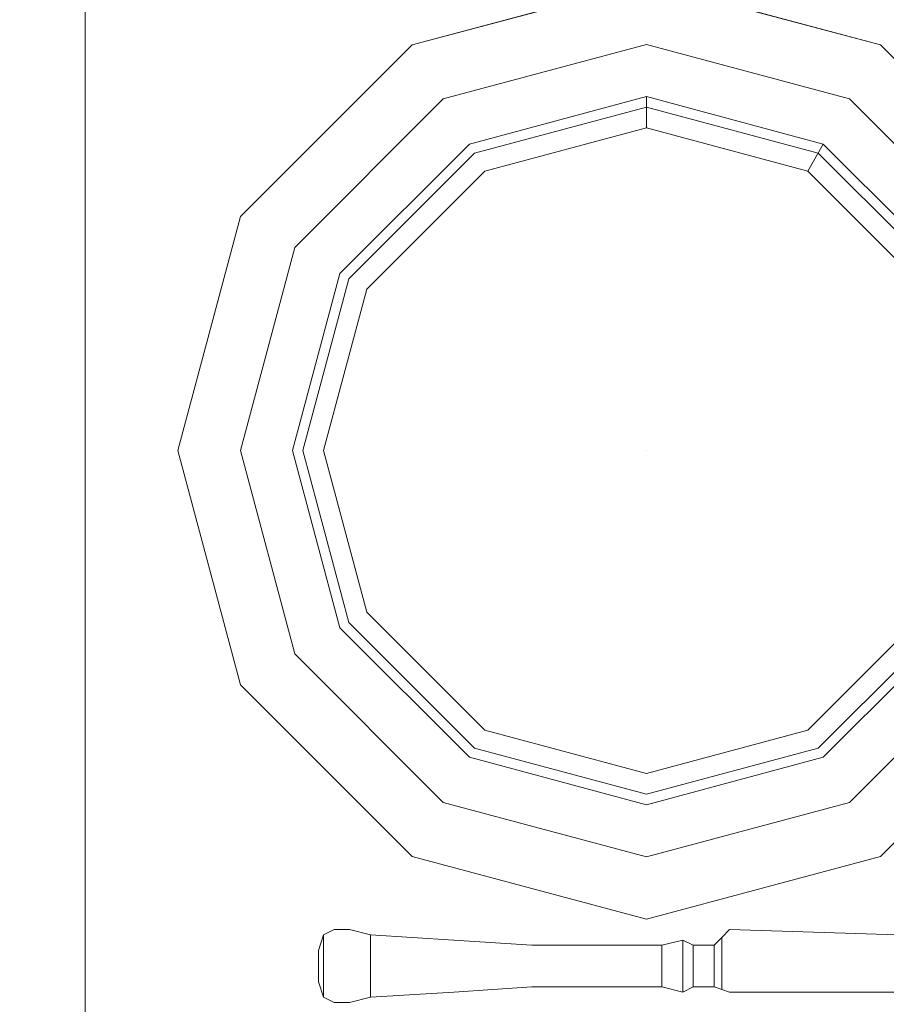
# Model space of a CAD drawing. Units: inches. Extents: x 375 to 1122, y 27 to 1069.
# Tile 38 of 155: x 705.14 to 715.39, y 296.54 to 308.18. Entities that reach past the tile are written whole.
import ezdxf

# ---------------------------------------------------------------- set-up
doc = ezdxf.new("R2010")
doc.units = ezdxf.units.IN
doc.layers.add('A-ANNO-DIMS', color=2, linetype='Continuous', lineweight=18)
doc.layers.add('Furniture', color=30, linetype='Continuous', lineweight=18)
doc.styles.get("Standard").update_dxf_attribs({"font": 'arial.ttf'})
doc.dimstyles.new('ISO-25', dxfattribs={"dimtxt": 12, "dimasz": 2.5, "dimexe": 1.5, "dimexo": 1.5, "dimtad": 1, "dimdec": 1, "dimlunit": 3, "dimtxsty": 'Standard', "dimblk": 'ARCHTICK', "dimcen": 2.5, "dimadec": 0, "dimazin": 0, "dimtfac": 1, "dimtdec": 1, "dimtmove": 0, "dimatfit": 3, "dimfxl": 1.5, "dimfxlon": 1, "dimarcsym": 0})

# ---------------------------------------------------------------- blocks, each defined once
blk = doc.blocks.new('A$C403C54AD')
blk.add_line((0.83575, 0.52421, -0.0006), (1.99923, 0.52421, -0.0006))
at = {"linetype": 'ByBlock'}
for points, invisible_edges in [([(1.01094, 0.81008, -0.00874), (1.02018, 0.79408, -0.00874), (0.97623, 0.75014, -0.00874), (0.96024, 0.75938, -0.00874)], 5), ([(1.02787, 0.78075, -0.02259), (1.01094, 0.81008, -0.01335), (0.96024, 0.75938, -0.01335), (0.98956, 0.74244, -0.02259)], 5), ([(1.17085, 0.74244, -0.02259), (1.20017, 0.75938, -0.01335), (1.14947, 0.81008, -0.01335), (1.13254, 0.78075, -0.02259)], 5), ([(1.20017, 0.75938, -0.00874), (1.18418, 0.75014, -0.00874), (1.14023, 0.79408, -0.00874), (1.14947, 0.81008, -0.00874)], 5), ([(1.02018, 0.79408, -0.00874), (1.02941, 0.77809, -0.01489), (0.99223, 0.74091, -0.01489), (0.97623, 0.75014, -0.00874)], 5), ([(1.18418, 0.75014, -0.00874), (1.16818, 0.74091, -0.01489), (1.131, 0.77809, -0.01489), (1.14023, 0.79408, -0.00874)], 5), ([(1.0802, 0.7917, -0.01489), (1.0802, 0.69011, -0.01489), (1.0802, 0.69011, -0.01489), (1.02941, 0.77809, -0.01489)], 5), ([(1.131, 0.77809, -0.01489), (1.0802, 0.69011, -0.01489), (1.0802, 0.69011, -0.01489), (1.0802, 0.7917, -0.01489)], 5), ([(1.03249, 0.77276, -0.03183), (1.02787, 0.78075, -0.02259), (0.98956, 0.74244, -0.02259), (0.99756, 0.73783, -0.03183)], 1), ([(1.16285, 0.73783, -0.03183), (1.17085, 0.74244, -0.02259), (1.13254, 0.78075, -0.02259), (1.12792, 0.77276, -0.03183)], 5), ([(1.02941, 0.77809, -0.01489), (1.0802, 0.69011, -0.01489), (1.0802, 0.69011, -0.01489), (0.99223, 0.74091, -0.01489)], 5), ([(1.16818, 0.74091, -0.01489), (1.0802, 0.69011, -0.01489), (1.0802, 0.69011, -0.01489), (1.131, 0.77809, -0.01489)], 5), ([(0.96024, 0.75938, -0.00874), (0.97623, 0.75014, -0.00874), (0.96015, 0.69011, -0.00874), (0.94168, 0.69011, -0.00874)], 5), ([(0.98956, 0.74244, -0.02259), (0.96024, 0.75938, -0.01335), (0.94168, 0.69011, -0.01335), (0.97554, 0.69011, -0.02259)], 5), ([(1.18487, 0.69011, -0.02259), (1.21873, 0.69011, -0.01335), (1.20017, 0.75938, -0.01335), (1.17085, 0.74244, -0.02259)], 5), ([(1.21873, 0.69011, -0.00874), (1.20026, 0.69011, -0.00874), (1.18418, 0.75014, -0.00874), (1.20017, 0.75938, -0.00874)], 5), ([(0.97623, 0.75014, -0.00874), (0.99223, 0.74091, -0.01489), (0.97862, 0.69011, -0.01489), (0.96015, 0.69011, -0.00874)], 5), ([(1.20026, 0.69011, -0.00874), (1.18179, 0.69011, -0.01489), (1.16818, 0.74091, -0.01489), (1.18418, 0.75014, -0.00874)], 5), ([(1.17563, 0.69011, -0.03183), (1.18487, 0.69011, -0.02259), (1.17085, 0.74244, -0.02259), (1.16285, 0.73783, -0.03183)], 5), ([(0.99223, 0.74091, -0.01489), (1.0802, 0.69011, -0.01489), (1.0802, 0.69011, -0.01489), (0.97862, 0.69011, -0.01489)], 5), ([(1.18179, 0.69011, -0.01489), (1.0802, 0.69011, -0.01489), (1.0802, 0.69011, -0.01489), (1.16818, 0.74091, -0.01489)], 5), ([(0.94168, 0.69011, -0.00874), (0.96015, 0.69011, -0.00874), (0.97623, 0.63008, -0.00874), (0.96024, 0.62085, -0.00874)], 5), ([(0.97554, 0.69011, -0.02259), (0.94168, 0.69011, -0.01335), (0.96024, 0.62085, -0.01335), (0.98956, 0.63778, -0.02259)], 5), ([(0.96015, 0.69011, -0.00874), (0.97862, 0.69011, -0.01489), (0.99223, 0.63932, -0.01489), (0.97623, 0.63008, -0.00874)], 5), ([(0.98477, 0.69011, -0.03183), (0.97554, 0.69011, -0.02259), (0.98956, 0.63778, -0.02259), (0.99756, 0.6424, -0.03183)], 4), ([(0.97862, 0.69011, -0.01489), (1.0802, 0.69011, -0.01489), (1.0802, 0.69011, -0.01489), (0.99223, 0.63932, -0.01489)], 5), ([(0.99223, 0.63932, -0.01489), (1.0802, 0.69011, -0.01489), (1.0802, 0.69011, -0.01489), (1.02941, 0.60214, -0.01489)], 5), ([(1.02941, 0.60214, -0.01489), (1.0802, 0.69011, -0.01489), (1.0802, 0.69011, -0.01489), (1.0802, 0.58853, -0.01489)], 5), ([(1.0802, 0.58853, -0.01489), (1.0802, 0.69011, -0.01489), (1.0802, 0.69011, -0.01489), (1.131, 0.60214, -0.01489)], 5), ([(1.131, 0.60214, -0.01489), (1.0802, 0.69011, -0.01489), (1.0802, 0.69011, -0.01489), (1.16818, 0.63932, -0.01489)], 5), ([(1.16818, 0.63932, -0.01489), (1.0802, 0.69011, -0.01489), (1.0802, 0.69011, -0.01489), (1.18179, 0.69011, -0.01489)], 5), ([(1.16285, 0.6424, -0.03183), (1.17085, 0.63778, -0.02259), (1.18487, 0.69011, -0.02259), (1.17563, 0.69011, -0.03183)], 5), ([(1.18418, 0.63008, -0.00874), (1.16818, 0.63932, -0.01489), (1.18179, 0.69011, -0.01489), (1.20026, 0.69011, -0.00874)], 5), ([(1.17085, 0.63778, -0.02259), (1.20017, 0.62085, -0.01335), (1.21873, 0.69011, -0.01335), (1.18487, 0.69011, -0.02259)], 5), ([(1.20017, 0.62085, -0.00874), (1.18418, 0.63008, -0.00874), (1.20026, 0.69011, -0.00874), (1.21873, 0.69011, -0.00874)], 5), ([(0.99756, 0.6424, -0.03183), (0.98956, 0.63778, -0.02259), (1.02787, 0.59947, -0.02259), (1.03249, 0.60747, -0.03183)], 5), ([(1.12792, 0.60747, -0.03183), (1.13254, 0.59947, -0.02259), (1.17085, 0.63778, -0.02259), (1.16285, 0.6424, -0.03183)], 5), ([(0.98956, 0.63778, -0.02259), (0.96024, 0.62085, -0.01335), (1.01094, 0.57014, -0.01335), (1.02787, 0.59947, -0.02259)], 5), ([(0.97623, 0.63008, -0.00874), (0.99223, 0.63932, -0.01489), (1.02941, 0.60214, -0.01489), (1.02018, 0.58614, -0.00874)], 5), ([(1.14023, 0.58614, -0.00874), (1.131, 0.60214, -0.01489), (1.16818, 0.63932, -0.01489), (1.18418, 0.63008, -0.00874)], 5), ([(1.13254, 0.59947, -0.02259), (1.14947, 0.57014, -0.01335), (1.20017, 0.62085, -0.01335), (1.17085, 0.63778, -0.02259)], 5), ([(0.96024, 0.62085, -0.00874), (0.97623, 0.63008, -0.00874), (1.02018, 0.58614, -0.00874), (1.01094, 0.57014, -0.00874)], 5), ([(1.14947, 0.57014, -0.00874), (1.14023, 0.58614, -0.00874), (1.18418, 0.63008, -0.00874), (1.20017, 0.62085, -0.00874)], 5), ([(1.03249, 0.60747, -0.03183), (1.02787, 0.59947, -0.02259), (1.0802, 0.58545, -0.02259), (1.0802, 0.59468, -0.03183)], 5), ([(1.0802, 0.59468, -0.03183), (1.0802, 0.58545, -0.02259), (1.13254, 0.59947, -0.02259), (1.12792, 0.60747, -0.03183)], 5), ([(1.02018, 0.58614, -0.00874), (1.02941, 0.60214, -0.01489), (1.0802, 0.58853, -0.01489), (1.0802, 0.57006, -0.00874)], 5), ([(1.0802, 0.57006, -0.00874), (1.0802, 0.58853, -0.01489), (1.131, 0.60214, -0.01489), (1.14023, 0.58614, -0.00874)], 5), ([(1.02787, 0.59947, -0.02259), (1.01094, 0.57014, -0.01335), (1.0802, 0.55159, -0.01335), (1.0802, 0.58545, -0.02259)], 5), ([(1.0802, 0.58545, -0.02259), (1.0802, 0.55159, -0.01335), (1.14947, 0.57014, -0.01335), (1.13254, 0.59947, -0.02259)], 5), ([(1.01094, 0.57014, -0.00874), (1.02018, 0.58614, -0.00874), (1.0802, 0.57006, -0.00874), (1.0802, 0.55159, -0.00874)], 5), ([(1.0802, 0.55159, -0.00874), (1.0802, 0.57006, -0.00874), (1.14023, 0.58614, -0.00874), (1.14947, 0.57014, -0.00874)], 5)]:
    blk.add_3dface(points, dxfattribs=dict(at, invisible_edges=invisible_edges))
for points in [[(1.01094, 0.81008, -0.01335), (1.01094, 0.81008, -0.00874), (0.96024, 0.75938, -0.00874), (0.96024, 0.75938, -0.01335)], [(1.20017, 0.75938, -0.01335), (1.20017, 0.75938, -0.00874), (1.14947, 0.81008, -0.00874), (1.14947, 0.81008, -0.01335)], [(0.96024, 0.75938, -0.01335), (0.96024, 0.75938, -0.00874), (0.94168, 0.69011, -0.00874), (0.94168, 0.69011, -0.01335)], [(1.21873, 0.69011, -0.01335), (1.21873, 0.69011, -0.00874), (1.20017, 0.75938, -0.00874), (1.20017, 0.75938, -0.01335)], [(0.99756, 0.73783, -0.03183), (0.98956, 0.74244, -0.02259), (0.97554, 0.69011, -0.02259), (0.98477, 0.69011, -0.03183)], [(0.94168, 0.69011, -0.01335), (0.94168, 0.69011, -0.00874), (0.96024, 0.62085, -0.00874), (0.96024, 0.62085, -0.01335)], [(1.20017, 0.62085, -0.01335), (1.20017, 0.62085, -0.00874), (1.21873, 0.69011, -0.00874), (1.21873, 0.69011, -0.01335)], [(0.96024, 0.62085, -0.01335), (0.96024, 0.62085, -0.00874), (1.01094, 0.57014, -0.00874), (1.01094, 0.57014, -0.01335)], [(1.14947, 0.57014, -0.01335), (1.14947, 0.57014, -0.00874), (1.20017, 0.62085, -0.00874), (1.20017, 0.62085, -0.01335)], [(1.01094, 0.57014, -0.01335), (1.01094, 0.57014, -0.00874), (1.0802, 0.55159, -0.00874), (1.0802, 0.55159, -0.01335)], [(1.0802, 0.55159, -0.01335), (1.0802, 0.55159, -0.00874), (1.14947, 0.57014, -0.00874), (1.14947, 0.57014, -0.01335)]]:
    blk.add_3dface(points, dxfattribs=at)
for points, invisible_edges in [([(1.24028, 0.77323, -0.0249), (1.22489, 0.81171, -0.0249), (1.22181, 0.71474, -0.0249), (1.24028, 0.71474, -0.0249)], 5), ([(1.24028, 0.77323, -0.02644), (1.22489, 0.81171, -0.02644), (1.22181, 0.71474, -0.02644), (1.24028, 0.71474, -0.02644)], 5), ([(1.22489, 0.81171, -0.02644), (1.22489, 0.81171, -0.0249), (1.22181, 0.71474, -0.0249), (1.22181, 0.71474, -0.02644)], 5), ([(1.24028, 0.71474, -0.0249), (1.24028, 0.71474, -0.02644), (1.24028, 0.77323, -0.02644), (1.24028, 0.77323, -0.0249)], 5), ([(1.22181, 0.71474, -0.0249), (1.24028, 0.71474, -0.0249), (1.23951, 0.71243, -0.02413), (1.22412, 0.71243, -0.02413)], 1), ([(1.22181, 0.71474, -0.02644), (1.24028, 0.71474, -0.02644), (1.23951, 0.71243, -0.02721), (1.22412, 0.71243, -0.02721)], 1), ([(1.22181, 0.71474, -0.02644), (1.22181, 0.71474, -0.0249), (1.22412, 0.71243, -0.02413), (1.22412, 0.71243, -0.02721)], 5), ([(1.23951, 0.71243, -0.02721), (1.23951, 0.71243, -0.02413), (1.24028, 0.71474, -0.0249), (1.24028, 0.71474, -0.02644)], 5), ([(1.22412, 0.71243, -0.02413), (1.22412, 0.71243, -0.02721), (1.22643, 0.71012, -0.03029), (1.22643, 0.71012, -0.02105)], 5), ([(1.23874, 0.71012, -0.02105), (1.23874, 0.71012, -0.03029), (1.23951, 0.71243, -0.02721), (1.23951, 0.71243, -0.02413)], 5), ([(1.22643, 0.71012, -0.03029), (1.22643, 0.71012, -0.02105), (1.22643, 0.70396, -0.02105), (1.22643, 0.70396, -0.03029)], 1), ([(1.23874, 0.70396, -0.03029), (1.23874, 0.70396, -0.02105), (1.23874, 0.71012, -0.02105), (1.23874, 0.71012, -0.03029)], 4), ([(1.22643, 0.69473, -0.02105), (1.23874, 0.69473, -0.02105), (1.23874, 0.65625, -0.01951), (1.22643, 0.65625, -0.01951)], 4), ([(1.22643, 0.69473, -0.03029), (1.23874, 0.69473, -0.03029), (1.23874, 0.65625, -0.03183), (1.22643, 0.65625, -0.03183)], 4), ([(1.23874, 0.65625, -0.01951), (1.22643, 0.65625, -0.01951), (1.22489, 0.63316, -0.01951), (1.24028, 0.63316, -0.01951)], 5), ([(1.23874, 0.65625, -0.03183), (1.22643, 0.65625, -0.03183), (1.22489, 0.63316, -0.03183), (1.24028, 0.63316, -0.03183)], 5), ([(1.22489, 0.63316, -0.01951), (1.24028, 0.63316, -0.01951), (1.24182, 0.60854, -0.02105), (1.22335, 0.60854, -0.02105)], 1), ([(1.22489, 0.63316, -0.03183), (1.24028, 0.63316, -0.03183), (1.24182, 0.60854, -0.03029), (1.22335, 0.60854, -0.03029)], 1), ([(1.24182, 0.60854, -0.02105), (1.22335, 0.60854, -0.02105), (1.22181, 0.60238, -0.01951), (1.24336, 0.60238, -0.01951)], 4), ([(1.24182, 0.60854, -0.03029), (1.22335, 0.60854, -0.03029), (1.22181, 0.60238, -0.03183), (1.24336, 0.60238, -0.03183)], 4), ([(1.22181, 0.60238, -0.01951), (1.24336, 0.60238, -0.01951), (1.24336, 0.59776, -0.02105), (1.22181, 0.59776, -0.02105)], 5), ([(1.22181, 0.60238, -0.03183), (1.24336, 0.60238, -0.03183), (1.24336, 0.59776, -0.03029), (1.22181, 0.59776, -0.03029)], 5), ([(1.24336, 0.59776, -0.02105), (1.22181, 0.59776, -0.02105), (1.22335, 0.59468, -0.02259), (1.24182, 0.59468, -0.02259)], 1), ([(1.24336, 0.59776, -0.03029), (1.22181, 0.59776, -0.03029), (1.22335, 0.59468, -0.02875), (1.24182, 0.59468, -0.02875)], 1)]:
    blk.add_3dface(points, dxfattribs=dict(invisible_edges=invisible_edges))
for points in [[(1.22412, 0.71243, -0.02413), (1.23951, 0.71243, -0.02413), (1.23874, 0.71012, -0.02105), (1.22643, 0.71012, -0.02105)], [(1.22412, 0.71243, -0.02721), (1.23951, 0.71243, -0.02721), (1.23874, 0.71012, -0.03029), (1.22643, 0.71012, -0.03029)], [(1.23874, 0.71012, -0.02105), (1.22643, 0.71012, -0.02105), (1.22643, 0.70396, -0.02105), (1.23874, 0.70396, -0.02105)], [(1.23874, 0.71012, -0.03029), (1.22643, 0.71012, -0.03029), (1.22643, 0.70396, -0.03029), (1.23874, 0.70396, -0.03029)], [(1.22643, 0.70396, -0.02105), (1.23874, 0.70396, -0.02105), (1.24028, 0.70089, -0.01951), (1.22489, 0.70089, -0.01951)], [(1.22643, 0.70396, -0.03029), (1.23874, 0.70396, -0.03029), (1.24028, 0.70089, -0.03183), (1.22489, 0.70089, -0.03183)], [(1.22643, 0.70396, -0.02105), (1.22643, 0.70396, -0.03029), (1.22489, 0.70089, -0.03183), (1.22489, 0.70089, -0.01951)], [(1.24028, 0.70089, -0.01951), (1.24028, 0.70089, -0.03183), (1.23874, 0.70396, -0.03029), (1.23874, 0.70396, -0.02105)], [(1.24028, 0.70089, -0.01951), (1.22489, 0.70089, -0.01951), (1.22643, 0.69473, -0.02105), (1.23874, 0.69473, -0.02105)], [(1.24028, 0.70089, -0.03183), (1.22489, 0.70089, -0.03183), (1.22643, 0.69473, -0.03029), (1.23874, 0.69473, -0.03029)], [(1.22489, 0.70089, -0.03183), (1.22489, 0.70089, -0.01951), (1.22643, 0.69473, -0.02105), (1.22643, 0.69473, -0.03029)], [(1.23874, 0.69473, -0.03029), (1.23874, 0.69473, -0.02105), (1.24028, 0.70089, -0.01951), (1.24028, 0.70089, -0.03183)], [(1.22643, 0.69473, -0.02105), (1.22643, 0.69473, -0.03029), (1.22643, 0.65625, -0.03183), (1.22643, 0.65625, -0.01951)], [(1.23874, 0.65625, -0.01951), (1.23874, 0.65625, -0.03183), (1.23874, 0.69473, -0.03029), (1.23874, 0.69473, -0.02105)], [(1.22643, 0.65625, -0.03183), (1.22643, 0.65625, -0.01951), (1.22489, 0.63316, -0.01951), (1.22489, 0.63316, -0.03183)], [(1.24028, 0.63316, -0.03183), (1.24028, 0.63316, -0.01951), (1.23874, 0.65625, -0.01951), (1.23874, 0.65625, -0.03183)], [(1.22489, 0.63316, -0.01951), (1.22489, 0.63316, -0.03183), (1.22335, 0.60854, -0.03029), (1.22335, 0.60854, -0.02105)], [(1.24182, 0.60854, -0.02105), (1.24182, 0.60854, -0.03029), (1.24028, 0.63316, -0.03183), (1.24028, 0.63316, -0.01951)], [(1.22335, 0.60854, -0.03029), (1.22335, 0.60854, -0.02105), (1.22181, 0.60238, -0.01951), (1.22181, 0.60238, -0.03183)], [(1.24336, 0.60238, -0.03183), (1.24336, 0.60238, -0.01951), (1.24182, 0.60854, -0.02105), (1.24182, 0.60854, -0.03029)], [(1.22181, 0.60238, -0.01951), (1.22181, 0.60238, -0.03183), (1.22181, 0.59776, -0.03029), (1.22181, 0.59776, -0.02105)], [(1.24336, 0.59776, -0.02105), (1.24336, 0.59776, -0.03029), (1.24336, 0.60238, -0.03183), (1.24336, 0.60238, -0.01951)], [(1.22181, 0.59776, -0.03029), (1.22181, 0.59776, -0.02105), (1.22335, 0.59468, -0.02259), (1.22335, 0.59468, -0.02875)], [(1.24182, 0.59468, -0.02259), (1.24182, 0.59468, -0.02875), (1.24336, 0.59776, -0.03029), (1.24336, 0.59776, -0.02105)], [(1.22335, 0.59468, -0.02259), (1.24182, 0.59468, -0.02259), (1.2372, 0.59314, -0.02567), (1.22797, 0.59314, -0.02567)], [(1.22335, 0.59468, -0.02259), (1.22335, 0.59468, -0.02875), (1.22797, 0.59314, -0.02567)], [(1.22335, 0.59468, -0.02875), (1.24182, 0.59468, -0.02875), (1.2372, 0.59314, -0.02567), (1.22797, 0.59314, -0.02567)], [(1.2372, 0.59314, -0.02567), (1.2372, 0.59314, -0.02567), (1.24182, 0.59468, -0.02259), (1.24182, 0.59468, -0.02875)]]:
    blk.add_3dface(points)
blk = doc.blocks.new('_ArchTick')
at = {"color": 0, "linetype": 'ByBlock', "const_width": 0.15}
blk.add_lwpolyline([(-0.5, -0.5), (0.5, 0.5)], dxfattribs=at)
blk = doc.blocks.new('*D59')
at = {"layer": 'A-ANNO-DIMS', "color": 0, "lineweight": -2, "transparency": 16777216}
for p, q in [((668.717, 346.851), (665.717, 346.851)), ((667.217, 346.851), (667.217, 232.348)), ((668.717, 232.348), (665.717, 232.348)), ((667.217, 232.348), (667.217, 27.496))]:
    blk.add_line(p, q, dxfattribs=at)
at = {"layer": 'Defpoints', "color": 0, "transparency": 16777216}
for p in [(684.392, 346.851), (667.217, 232.348), (684.392, 232.348)]:
    blk.add_point(p, dxfattribs=at)
at = {"layer": 'A-ANNO-DIMS', "color": 0, "lineweight": -2, "transparency": 16777216, "xscale": 2.5, "yscale": 2.5, "zscale": 2.5}
for p, rotation in [((667.217, 346.851), 90), ((667.217, 232.348), 270)]:
    blk.add_blockref('_ArchTick', p, dxfattribs=dict(at, rotation=rotation))
at = {"layer": 'A-ANNO-DIMS', "color": 0, "transparency": 16777216, "insert": (660.387, 128.672), "char_height": 12, "attachment_point": 5, "rotation": 90}
blk.add_mtext('DINING SET 9\'-6 1/2" TYP.', dxfattribs=at)

msp = doc.modelspace()

# ---------------------------------------------------------------- block references
at = {"layer": 'Furniture', "xscale": 39.9918517141215, "yscale": 39.9918517141215, "zscale": 39.9918517141215, "rotation": 270}
msp.add_blockref('A$C403C54AD', (684.955, 346.287, 0.024), dxfattribs=at)

# ---------------------------------------------------------------- dimensions: what is measured, and where the dimension line sits
at = {"layer": 'A-ANNO-DIMS'}
dim = msp.add_linear_dim(base=(667.217, 232.348), p1=(684.392, 346.851), p2=(684.392, 232.348), angle=270, text='DINING SET <> TYP.', dimstyle='ISO-25', override={"dimdec": 1, "dimlfac": 1, "dimrnd": 0, "dimzin": 1, "dimdsep": 46, "dimlunit": 4, "dimfrac": 2}, dxfattribs=at)
dim.commit()
dim.dimension.update_dxf_attribs({"geometry": '*D59', "text_midpoint": (660.387, 128.672)})

doc.saveas('drawing.dxf')
